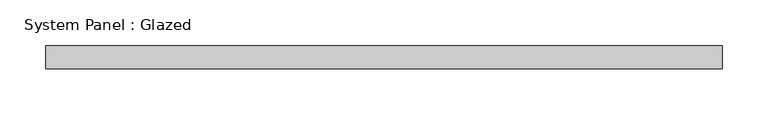
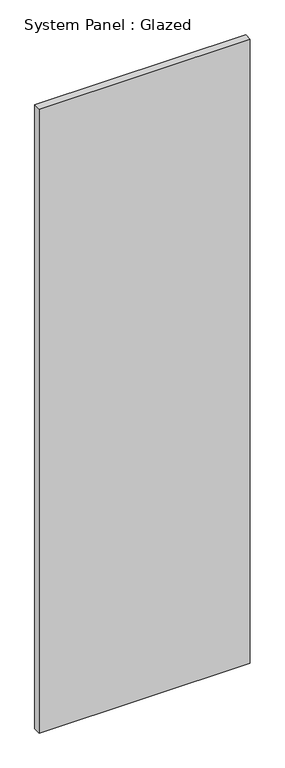
"""IFC4 building model written with IfcOpenShell, lengths in millimetres: plate geometry, System Panel : Glazed."""

from ifc_helpers import new_model, si_unit, origin, origin_with_axes, place, context, project, spatial, polyline, outline, extrude, source, transform, mapped, element, save


def system_panel_glazed_479de850(model_context):
    return source(origin(), model_context, "Body", "SweptSolid", [
        extrude(outline(polyline([(371.475, 19.05), (-371.475, 19.05), (-371.475, 44.45), (371.475, 44.45), (371.475, 19.05)])), origin_with_axes(), (0.0, 0.0, 1.0), 2318.7520936),
    ])


if __name__ == "__main__":
    model = new_model("IFC4")
    model_context = context("Model", 3, world=origin())
    ifc_project = project(units=[si_unit("LENGTHUNIT", "METRE", prefix="MILLI")], contexts=[model_context])
    site = spatial("IfcSite", under=ifc_project)
    building = spatial("IfcBuilding", under=site)
    placement = place(None, origin())
    system_panel_glazed_shape = system_panel_glazed_479de850(model_context)
    element("IfcPlate", 1, ObjectType="System Panel : Glazed", at=placement, inside=building, context=model_context, shape_type="MappedRepresentation", body=[
        mapped(system_panel_glazed_shape, transform((0.0, 0.0, 0.0), x_axis=(1.0, 0.0, 0.0), y_axis=(0.0, 1.0, 0.0), z_axis=(0.0, 0.0, 1.0))),
    ])
    save(model, "model.ifc")

# Revit data of these elements
# Type "System Panel : Glazed"
#   Construction Type Id = "GSP4R"
#   Analytic Construction = "1/8 in Pilkington single glazing"
#   Visual Light Transmittance = 0.9
#   Solar Heat Gain Coefficient = 0.86
#   Heat Transfer Coefficient (U) = 1.18115 BTU/(h·ft²·°F)
#   Define Thermal Properties by = 1
# Element 1 (IfcPlate, "System Panel : Glazed")
#   Materials on its faces: "Glass"
# Materials
#   "Glass": class "Glass", colour RGB 0 128 192, transparency 0.75, Description = "Soda Lime Glass", Cost = 0
